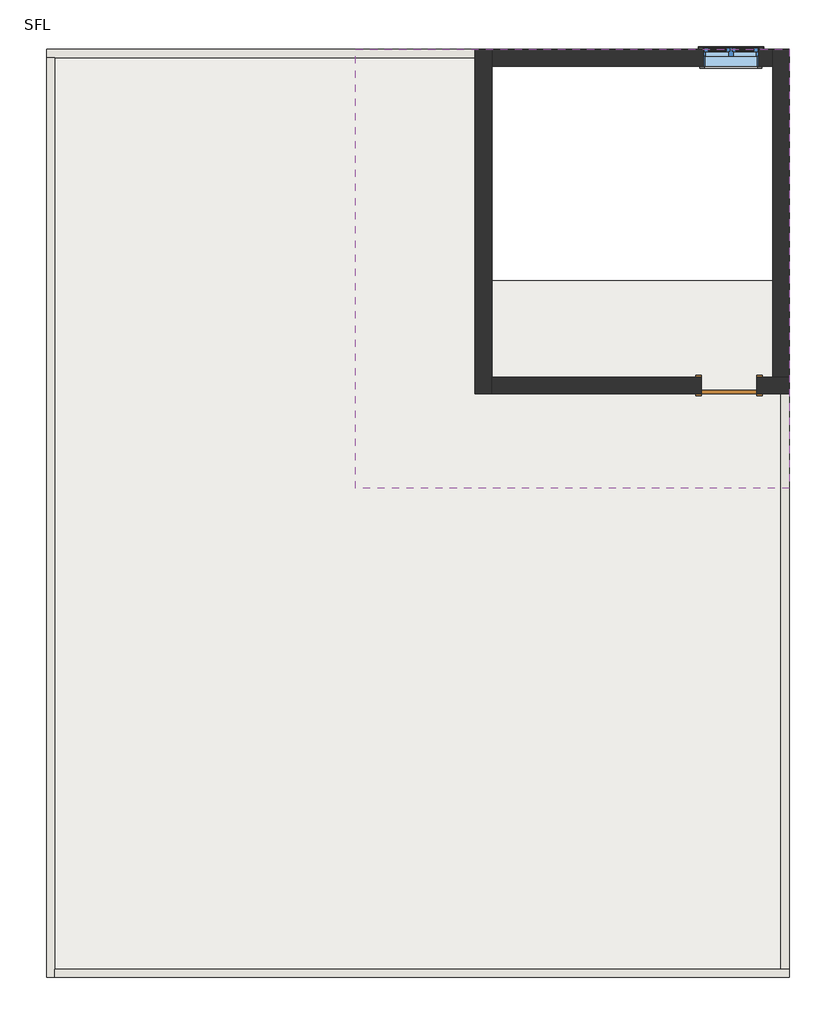
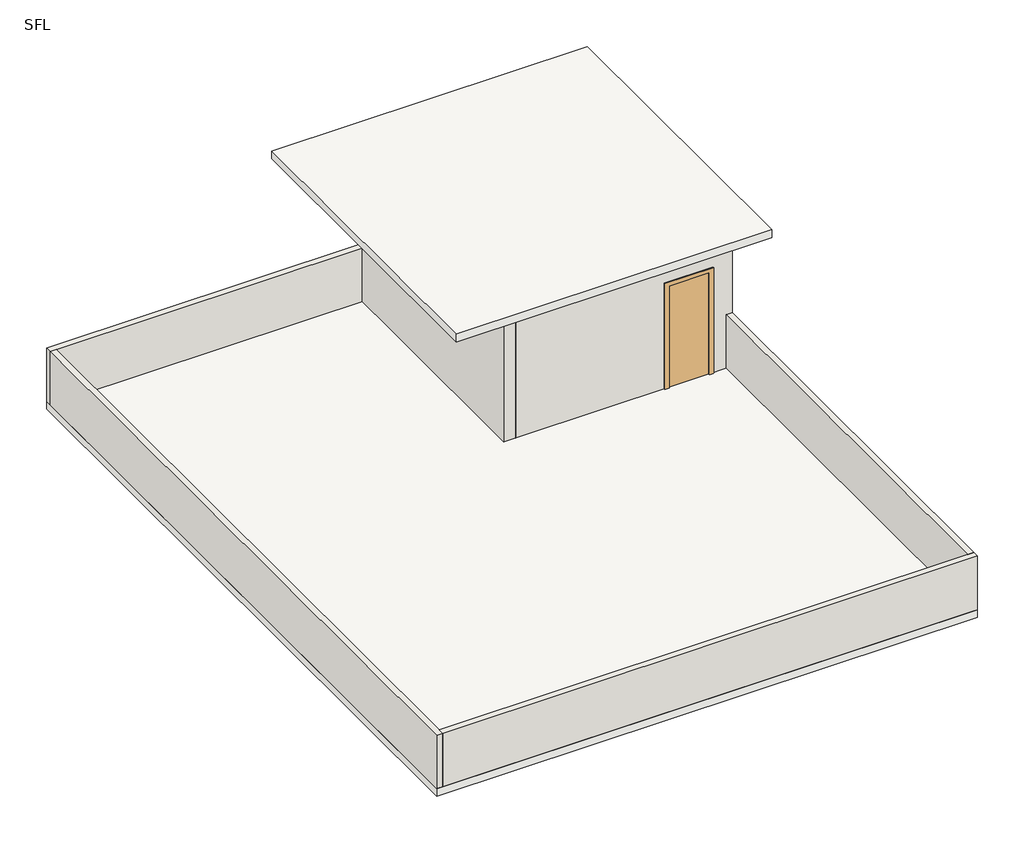
# One storey: 8 walls, 4 proxies, 2 slabs, 1 door, 1 window.
"""IFC4 building model written with IfcOpenShell, lengths in millimetres."""

from ifc_helpers import new_model, si_unit, frame, origin, place, context, project, spatial, polyline, outline, extrude, faceted_brep, transform, mapped, element, save
from components import muntin_pattern_2x2_muntin_pattern_2x2_1c12c043, muntin_pattern_2x2_muntin_pattern_2x2_88561ff7, trim_window_exterior_flat_with_sill_8633aa7b, trim_window_interior_flat_picture_frame_129e3d92, door_85036156, window_9dcce3b5

model = new_model("IFC4")

# Units and contexts
model_context = context("Model", 3, world=origin())
ifc_project = project(units=[si_unit("LENGTHUNIT", "METRE", prefix="MILLI")], contexts=[model_context])

# Site, building, storey
site = spatial("IfcSite", under=ifc_project)
building = spatial("IfcBuilding", under=site)
storey = spatial("IfcBuildingStorey", under=building, Name="SFL", Elevation=7010.4)

# Proxies
placement = place(None, origin())
muntin_pattern_2x2_muntin_pattern_2x2_shape = muntin_pattern_2x2_muntin_pattern_2x2_1c12c043(model_context)
element("IfcBuildingElementProxy", 1, Name="Muntin Pattern_2x2 : Muntin Pattern_2x2", ObjectType="Muntin Pattern_2x2 : Muntin Pattern_2x2", at=placement, inside=storey, context=model_context, shape_type="MappedRepresentation", body=[
    mapped(muntin_pattern_2x2_muntin_pattern_2x2_shape, transform((-4724.7382748, 12392.4878362, 7080.25), x_axis=(1.0, 0.0, 0.0), y_axis=(0.0, 1.0, 0.0), z_axis=(0.0, 0.0, 1.0))),
])
muntin_pattern_2x2_muntin_pattern_2x2_2_shape = muntin_pattern_2x2_muntin_pattern_2x2_88561ff7(model_context)
element("IfcBuildingElementProxy", 2, Name="Muntin Pattern_2x2 : Muntin Pattern_2x2", ObjectType="Muntin Pattern_2x2 : Muntin Pattern_2x2", at=placement, inside=storey, context=model_context, shape_type="MappedRepresentation", body=[
    mapped(muntin_pattern_2x2_muntin_pattern_2x2_2_shape, transform((-4346.9132748, 12392.4878362, 7080.25), x_axis=(-1.0, 0.0, 0.0), y_axis=(0.0, -1.0, 0.0), z_axis=(0.0, 0.0, 1.0))),
])
trim_window_exterior_flat_with_sill_shape = trim_window_exterior_flat_with_sill_8633aa7b(model_context)
element("IfcBuildingElementProxy", 3, Name="Trim-Window-Exterior-Flat : with Sill", ObjectType="Trim-Window-Exterior-Flat : with Sill", at=placement, inside=storey, context=model_context, shape_type="MappedRepresentation", body=[
    mapped(trim_window_exterior_flat_with_sill_shape, transform((-4535.8257748, 12402.0128362, 8686.8), x_axis=(-1.0, 0.0, 0.0), y_axis=(0.0, 0.0, 1.0), z_axis=(0.0, 1.0, 0.0))),
])
trim_window_interior_flat_picture_frame_shape = trim_window_interior_flat_picture_frame_129e3d92(model_context)
element("IfcBuildingElementProxy", 4, Name="Trim-Window-Interior-Flat : Picture Frame", ObjectType="Trim-Window-Interior-Flat : Picture Frame", at=placement, inside=storey, context=model_context, shape_type="MappedRepresentation", body=[
    mapped(trim_window_interior_flat_picture_frame_shape, transform((-4535.8257748, 12173.4128362, 8686.8), x_axis=(1.0, 0.0, 0.0), y_axis=(0.0, 0.0, 1.0), z_axis=(0.0, -1.0, 0.0))),
])

# Door
door_shape = door_85036156(model_context)
element("IfcDoor", 5, ObjectType="Single-Flush : 30\" x 80\"", at=placement, inside=storey, context=model_context, shape_type="MappedRepresentation", body=[
    mapped(door_shape, transform((-4561.2257748, 7791.9128362, 7010.4), x_axis=(1.0, 0.0, 0.0), y_axis=(0.0, 1.0, 0.0), z_axis=(0.0, 0.0, 1.0))),
])

# Slabs
element("IfcSlab", 6, ObjectType="6\"", at=placement, inside=storey, context=model_context, shape_type="SweptSolid", body=[
    extrude(outline(polyline([(-3735.7257748, 12402.0128362), (-3735.7257748, -321.0059138), (-13924.3002526, -321.0059138), (-13924.3002526, 12402.0128362), (-3735.7257748, 12402.0128362)]), holes=[polyline([(-3967.5002526, 12173.4128362), (-7815.6002526, 12173.4128362), (-7815.6002526, 9239.7128362), (-3967.5002526, 9239.7128362), (-3967.5002526, 12173.4128362)])]), frame((0.0, 0.0, 6858.0), z_axis=(0.0, 0.0, 1.0), x_axis=(1.0, 0.0, 0.0)), (0.0, 0.0, 1.0), 152.4),
])
element("IfcSlab", 7, ObjectType="6\"", at=placement, inside=storey, context=model_context, shape_type="SweptSolid", body=[
    extrude(outline(polyline([(-3735.7257748, 6382.2128362), (-9682.5002526, 6382.2128362), (-9682.5002526, 12402.0128362), (-3735.7257748, 12402.0128362), (-3735.7257748, 6382.2128362)])), frame((0.0, 0.0, 10363.2), z_axis=(0.0, 0.0, 1.0), x_axis=(1.0, 0.0, 0.0)), (0.0, 0.0, 1.0), 152.4),
])

# Walls
element("IfcWall", 8, ObjectType="10\"", at=placement, inside=storey, context=model_context, shape_type="Brep", body=[
    faceted_brep([(-8044.2002526, 12402.0128362, 10363.2), (-8044.2002526, 12402.0128362, 8077.2), (-8044.2002526, 12402.0128362, 7010.4), (-8044.2002526, 12287.7128362, 7010.4), (-8044.2002526, 7677.6128362, 7010.4), (-8044.2002526, 7677.6128362, 10363.2), (-7815.6002526, 12402.0128362, 7010.4), (-7815.6002526, 12402.0128362, 10363.2), (-7815.6002526, 12173.4128362, 10363.2), (-7815.6002526, 7906.2128362, 10363.2), (-7815.6002526, 7677.6128362, 10363.2), (-7815.6002526, 7677.6128362, 7010.4), (-7815.6002526, 7906.2128362, 7010.4), (-7815.6002526, 12173.4128362, 7010.4)], [[[0, 1, 2, 3, 4, 5]], [[6, 7, 8, 9, 10, 11, 12, 13]], [[4, 3, 2, 6, 13, 12, 11]], [[0, 5, 10, 9, 8, 7]], [[5, 4, 11, 10]], [[0, 7, 6, 2, 1]]]),
])
element("IfcWall", 9, ObjectType="10\"", at=placement, inside=storey, context=model_context, shape_type="Brep", body=[
    faceted_brep([(-4180.2257748, 7677.6128362, 9042.4), (-4180.2257748, 7677.6128362, 7010.4), (-3850.0257748, 7677.6128362, 7010.4), (-3735.7257748, 7677.6128362, 7010.4), (-3735.7257748, 7677.6128362, 8077.2), (-3735.7257748, 7677.6128362, 10363.2), (-7815.6002526, 7677.6128362, 10363.2), (-7815.6002526, 7677.6128362, 7010.4), (-4942.2257748, 7677.6128362, 7010.4), (-4942.2257748, 7677.6128362, 9042.4), (-3735.7257748, 7906.2128362, 7010.4), (-3964.3257748, 7906.2128362, 7010.4), (-4180.2257748, 7906.2128362, 7010.4), (-4180.2257748, 7906.2128362, 9042.4), (-4942.2257748, 7906.2128362, 9042.4), (-4942.2257748, 7906.2128362, 7010.4), (-7815.6002526, 7906.2128362, 7010.4), (-7815.6002526, 7906.2128362, 10363.2), (-3964.3257748, 7906.2128362, 10363.2), (-3735.7257748, 7906.2128362, 10363.2)], [[[0, 1, 2, 3, 4, 5, 6, 7, 8, 9]], [[10, 11, 12, 13, 14, 15, 16, 17, 18, 19]], [[8, 7, 16, 15]], [[3, 2, 1, 12, 11, 10]], [[6, 5, 19, 18, 17]], [[7, 6, 17, 16]], [[13, 12, 1, 0]], [[14, 13, 0, 9]], [[15, 14, 9, 8]], [[3, 10, 19, 5, 4]]]),
])
element("IfcWall", 10, ObjectType="10\"", at=placement, inside=storey, context=model_context, shape_type="Brep", body=[
    faceted_brep([(-3735.7257748, 7906.2128362, 10363.2), (-3735.7257748, 7906.2128362, 7010.4), (-3735.7257748, 12402.0128362, 7010.4), (-3735.7257748, 12402.0128362, 10363.2), (-3964.3257748, 7906.2128362, 7010.4), (-3964.3257748, 7906.2128362, 10363.2), (-3964.3257748, 12173.4128362, 10363.2), (-3964.3257748, 12402.0128362, 10363.2), (-3964.3257748, 12402.0128362, 7010.4), (-3964.3257748, 12173.4128362, 7010.4)], [[[0, 1, 2, 3]], [[4, 5, 6, 7, 8, 9]], [[2, 1, 4, 9, 8]], [[0, 3, 7, 6, 5]], [[3, 2, 8, 7]], [[0, 5, 4, 1]]]),
])
element("IfcWall", 11, ObjectType="10\"", at=placement, inside=storey, context=model_context, shape_type="SweptSolid", body=[
    extrude(outline(polyline([(7010.4, -7815.6002526), (7010.4, -4916.8257748), (8686.8, -4916.8257748), (8686.8, -4154.8257748), (7010.4, -4154.8257748), (7010.4, -3964.3257748), (10363.2, -3964.3257748), (10363.2, -7815.6002526), (7010.4, -7815.6002526)])), frame((0.0, 12173.4128362, 0.0), z_axis=(0.0, 1.0, 0.0), x_axis=(0.0, 0.0, 1.0)), (0.0, 0.0, 1.0), 228.6),
])
element("IfcWall", 12, ObjectType="5\"", at=placement, inside=storey, context=model_context, shape_type="Brep", body=[
    faceted_brep([(-8044.2002526, 12402.0128362, 7010.4), (-13924.3002526, 12402.0128362, 7010.4), (-13924.3002526, 12402.0128362, 8077.2), (-8044.2002526, 12402.0128362, 8077.2), (-8044.2002526, 12287.7128362, 7010.4), (-8044.2002526, 12287.7128362, 8077.2), (-13810.0002526, 12287.7128362, 8077.2), (-13924.3002526, 12287.7128362, 8077.2), (-13924.3002526, 12287.7128362, 7010.4), (-13810.0002526, 12287.7128362, 7010.4)], [[[0, 1, 2, 3]], [[4, 5, 6, 7, 8, 9]], [[1, 0, 4, 9, 8]], [[3, 2, 7, 6, 5]], [[0, 3, 5, 4]], [[2, 1, 8, 7]]]),
])
element("IfcWall", 13, ObjectType="5\"", at=placement, inside=storey, context=model_context, shape_type="Brep", body=[
    faceted_brep([(-13924.3002526, 12287.7128362, 7010.4), (-13924.3002526, -321.0059138, 7010.4), (-13924.3002526, -321.0059138, 8077.2), (-13924.3002526, 12287.7128362, 8077.2), (-13810.0002526, 12287.7128362, 7010.4), (-13810.0002526, 12287.7128362, 8077.2), (-13810.0002526, -206.7059138, 8077.2), (-13810.0002526, -321.0059138, 8077.2), (-13810.0002526, -321.0059138, 7010.4), (-13810.0002526, -206.7059138, 7010.4)], [[[0, 1, 2, 3]], [[4, 5, 6, 7, 8, 9]], [[1, 0, 4, 9, 8]], [[3, 2, 7, 6, 5]], [[0, 3, 5, 4]], [[2, 1, 8, 7]]]),
])
element("IfcWall", 14, ObjectType="5\"", at=placement, inside=storey, context=model_context, shape_type="Brep", body=[
    faceted_brep([(-13810.0002526, -321.0059138, 7010.4), (-3735.7257748, -321.0059138, 7010.4), (-3735.7257748, -321.0059138, 8077.2), (-13810.0002526, -321.0059138, 8077.2), (-13810.0002526, -206.7059138, 7010.4), (-13810.0002526, -206.7059138, 8077.2), (-3850.0257748, -206.7059138, 8077.2), (-3735.7257748, -206.7059138, 8077.2), (-3735.7257748, -206.7059138, 7010.4), (-3850.0257748, -206.7059138, 7010.4)], [[[0, 1, 2, 3]], [[4, 5, 6, 7, 8, 9]], [[1, 0, 4, 9, 8]], [[3, 2, 7, 6, 5]], [[0, 3, 5, 4]], [[2, 1, 8, 7]]]),
])
element("IfcWall", 15, ObjectType="5\"", at=placement, inside=storey, context=model_context, shape_type="SweptSolid", body=[
    extrude(outline(polyline([(-3735.7257748, 7677.6128362), (-3735.7257748, -206.7059138), (-3850.0257748, -206.7059138), (-3850.0257748, 7677.6128362), (-3735.7257748, 7677.6128362)])), frame((0.0, 0.0, 7010.4), z_axis=(0.0, 0.0, 1.0), x_axis=(1.0, 0.0, 0.0)), (0.0, 0.0, 1.0), 1066.8),
])

# Window
window_shape = window_9dcce3b5(model_context)
element("IfcWindow", 16, ObjectType="Window-Casement-Double : 2'-6\" X 5'-6\"", at=placement, inside=storey, context=model_context, shape_type="MappedRepresentation", body=[
    mapped(window_shape, transform((-4535.8257748, 12287.7128362, 6096.0), x_axis=(1.0, 0.0, 0.0), y_axis=(0.0, 1.0, 0.0), z_axis=(0.0, 0.0, 1.0))),
])

save(model, "model.ifc")

# Revit data of these elements
# Type "Muntin Pattern_2x2 : Muntin Pattern_2x2"
#   Width [instance default] = 4' - 0"
#   Thickness = 0' - 0 1/2"
#   Height [instance default] = 4' - 0"
#   Distance = 0' - 0 3/4"
#   Interior Material [instance default] = none
#   Exterior Material [instance default] = none
#   Default Elevation = 0
# Type "Trim-Window-Exterior-Flat : with Sill"
#   Trim Width = 0' - 2 1/4"
#   Trim Thickness_Picture Frame = 0' - 1 1/4"
#   Trim Thickness_with Sill = 0' - 0 3/4"
#   Sill Thickness = 0' - 1 1/4"
#   Opening Width [instance default] = 2' - 0"
#   Opening Height [instance default] = 3' - 0"
#   Default Elevation = 4' - 0"
#   Sill = yes
#   Picture Frame = no
#   Trim Material [instance default] = none
# Type "Trim-Window-Interior-Flat : Picture Frame"
#   Trim Thickness_Picture Frame = 0' - 1 1/4"
#   Trim Width = 0' - 2 1/4"
#   Trim Thickness_with Sill = 0' - 0 3/4"
#   Sill Thickness = 0' - 1 1/4"
#   Opening Width [instance default] = 2' - 0"
#   Opening Height [instance default] = 3' - 0"
#   Default Elevation = 4' - 0"
#   Sill = no
#   Picture Frame = yes
#   Trim Material [instance default] = none
# Type "Single-Flush : 30\" x 80\""
#   Type Mark = "5"
#   Construction Type Id = "MDOOR"
#   Assembly Code = "C1020"
#   Analytic Construction = "Metal"
#   Thickness = 0' - 2"
#   Heat Transfer Coefficient (U) = 0.651978 BTU/(h·ft²·°F)
#   Height = 6' - 8"
#   Trim Projection Ext = 0' - 1"
#   Trim Projection Int = 0' - 1"
#   Trim Width = 0' - 3"
#   Width = 2' - 6"
#   Define Thermal Properties by = 1
#   Define Thermal Properties by = 1
#   Door Material = Door - Panel
#   Frame Material = Door - Frame
#   Visual Light Transmittance = 0
#   Solar Heat Gain Coefficient = 0
#   Function = (empty or 0)
#   Wall Closure = (empty or 0)
# Type "6\""
#   Assembly Code = "B1010"
#   Function = 0
#   Layers, outside or top first: 0' - 6" "Gypsum Wall Board" (function 1)
# Type "10\""
#   Assembly Code = "B2010"
#   Layers, outside or top first: 0' - 9" "Gypsum Wall Board" (function 1)
# Type "5\""
#   Assembly Code = "B2010"
#   Layers, outside or top first: 0' - 4 1/2" "Gypsum Wall Board" (function 1)
# Type "Window-Casement-Double : 2'-6\" X 5'-6\""
#   Type Mark = "21"
#   Fire Rating = "0.5h"
#   Assembly Code = "B2020100"
#   Analytic Construction = "Double glazing - domestic"
#   Frame Extension [instance default] = 0' - 0 1/4"
#   Window Inset [instance default] = 0' - 0"
#   Wall Thickness [instance default] = 0' - 6"
#   Interior Wall Closure [instance default] = 0' - 2 1/4"
#   Half Width = 1' - 3"
#   Visual Light Transmittance = 0.81
#   Thermal Resistance (R) = 1.8146 (h·ft²·°F)/BTU
#   Solar Heat Gain Coefficient = 0.76
#   Rough Width = 2' - 6 1/2"
#   Rough Height = 5' - 6 1/2"
#   Height = 5' - 6"
#   Heat Transfer Coefficient (U) = 0.5511 BTU/(h·ft²·°F)
#   Exterior Wall Closure [instance default] = 0' - 1 1/4"
#   Extension Jamb [instance default] = 0' - 2 1/4"
#   Default Sill Height = 3' - 0"
#   Width = 2' - 6"
#   Muntin Visibility = yes
#   Interior Trim Visibility [instance default] = yes
#   Exterior Trim Visibility [instance default] = yes
#   Extension Jamb Visibility [instance default] = yes
#   Interior Trim Material = Wood - Stained
#   Muntin Pattern = Muntin Pattern_2x2 : Muntin Pattern_2x2
#   Interior Trim = Trim-Window-Interior-Flat : Picture Frame
#   Interior Frame Material = Wood - Stained
#   Glass Panel Material = Glass
#   Exterior Trim Material = Clad - White
#   Exterior Trim = Trim-Window-Exterior-Flat : with Sill
#   Exterior Frame Material = Clad - White
#   Wall Closure = (empty or 0)
# Elements 1, 2 (IfcBuildingElementProxy, "Muntin Pattern_2x2 : Muntin Pattern_2x2")
#   Width = 0' - 9 5/8"
#   Height = 5' - 0 1/2"
#   Interior Material = Wood - Stained
#   Exterior Material = Clad - White
#   Phase Created = New Construction
#   Materials on its faces: "Clad - White", "Wood - Stained"
# Element 3 (IfcBuildingElementProxy, "Trim-Window-Exterior-Flat : with Sill")
#   Opening Width = 2' - 6"
#   Opening Height = 5' - 6"
#   Trim Material = Clad - White
#   Phase Created = New Construction
#   Materials on its faces: "Clad - White"
# Element 4 (IfcBuildingElementProxy, "Trim-Window-Interior-Flat : Picture Frame")
#   Opening Width = 2' - 6"
#   Opening Height = 5' - 6"
#   Trim Material = Wood - Stained
#   Phase Created = New Construction
#   Materials on its faces: "Wood - Stained"
# Element 5 (IfcDoor, "Single-Flush : 30\" x 80\"")
#   Phase Created = New Construction
#   Materials on its faces: "Door - Frame", "Door - Panel"
# Element 6 (IfcSlab, "6\"")
#   Height Offset From Level = 0' - 0"
#   Phase Created = New Construction
#   Materials on its faces: "Gypsum Wall Board"
# Element 7 (IfcSlab, "6\"")
#   Height Offset From Level = 11' - 6"
#   Phase Created = New Construction
#   Materials on its faces: "Gypsum Wall Board"
# Elements 8, 9, 10, 11 (IfcWall, "10\"")
#   Top Offset = 0' - 0"
#   Base Offset = 0' - 0"
#   Unconnected Height = 11' - 0"
#   wall height = 11' - 0"
#   Phase Created = New Construction
#   Base Constraint = SFL
#   Materials on its faces: "Gypsum Wall Board"
# Elements 12, 13, 14, 15 (IfcWall, "5\"")
#   Top Offset = 0' - 0"
#   Base Offset = 0' - 0"
#   Unconnected Height = 3' - 6"
#   wall height = 3' - 6"
#   Phase Created = New Construction
#   Base Constraint = SFL
#   Materials on its faces: "Gypsum Wall Board"
# Element 16 (IfcWindow, "Window-Casement-Double : 2'-6\" X 5'-6\"")
#   Mark = "22"
#   Window Inset = 0' - 0"
#   Interior Wall Closure = 0' - 2 1/4"
#   Frame Extension = 0' - 0 1/4"
#   Exterior Wall Closure = 0' - 1 1/4"
#   Interior Trim Visibility = yes
#   Exterior Trim Visibility = yes
#   Phase Created = New Construction
#   Materials on its faces: "Wood - Stained", "Glass", "Clad - White"
# Materials
#   "Door - Panel": class "Wood", colour RGB 210 159 95, transparency 0, Cost = 0
#   "Door - Frame": colour RGB 118 70 51, transparency 0, Cost = 0
#   "Gypsum Wall Board": class "Generic", colour RGB 228 228 228, transparency 0, Description = "Gypsum Wall Board", Cost = 0
#   "Wood - Stained": class "Wood", colour RGB 224 178 126, transparency 0, Cost = 0
#   "Glass": class "Glass", colour RGB 0 128 192, transparency 0.75, Description = "Soda Lime Glass", Cost = 0
#   "Clad - White": class "Wood", colour RGB 242 242 238, transparency 0, Cost = 0
